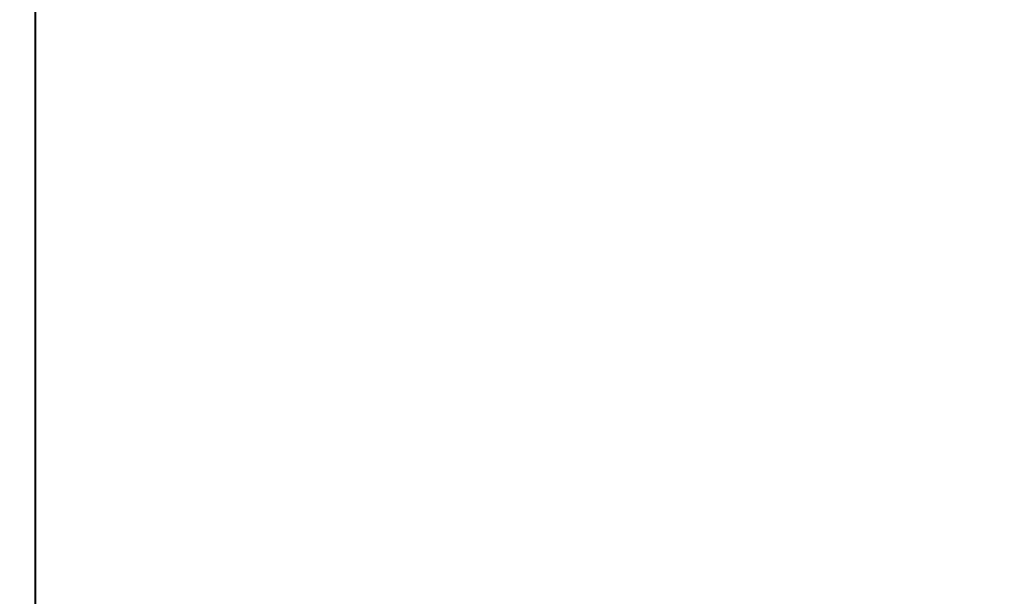
# Model space of a CAD drawing. Units: inches. Extents: x 459864 to 460310, y 324185 to 324787.
# Tile 83 of 112: x 460247.114882 to 460247.117712, y 324283.483832 to 324283.485489. Entities that reach past the tile are written whole.
import ezdxf

# ---------------------------------------------------------------- set-up
doc = ezdxf.new("R2010")
doc.units = ezdxf.units.IN
doc.layers.add('A-ANNO-DIMS', color=2, linetype='Continuous', lineweight=18)
doc.layers.add('A-WALL', color=7, linetype='Continuous', lineweight=40)
doc.styles.get("Standard").update_dxf_attribs({"font": 'arial.ttf'})
doc.dimstyles.new('ISO-25', dxfattribs={"dimtxt": 6, "dimasz": 2.5, "dimexe": 1.25, "dimexo": 0.625, "dimtad": 1, "dimdec": 1, "dimlunit": 3, "dimtxsty": 'Standard', "dimcen": 2.5, "dimadec": 0, "dimazin": 0, "dimtfac": 1, "dimtdec": 1, "dimtmove": 0, "dimatfit": 3, "dimfxl": 1, "dimarcsym": 0})

# ---------------------------------------------------------------- blocks, each defined once
blk = doc.blocks.new('*D21')
at = {"layer": 'A-ANNO-DIMS', "color": 0, "lineweight": -2, "transparency": 16777216}
for p, q in [((460247.7399266, 324715.4832328), (460309.5803685, 324715.4832328)), ((460308.3303685, 324712.9832328), (460308.3303685, 324285.9832328)), ((460247.7399266, 324283.4832328), (460309.5803685, 324283.4832328))]:
    blk.add_line(p, q, dxfattribs=at)
at = {"layer": 'A-ANNO-DIMS', "color": 0, "transparency": 16777216}
for points in [[(460307.9137019, 324712.9832328), (460308.7470352, 324712.9832328), (460308.3303685, 324715.4832328)], [(460307.9137019, 324285.9832328), (460308.7470352, 324285.9832328), (460308.3303685, 324283.4832328)]]:
    blk.add_solid(points, dxfattribs=at)
at = {"layer": 'Defpoints', "color": 0, "transparency": 16777216}
for p in [(460247.1149266, 324715.4832328), (460247.1149266, 324283.4832328), (460308.3303685, 324283.4832328)]:
    blk.add_point(p, dxfattribs=at)
at = {"layer": 'A-ANNO-DIMS', "color": 0, "transparency": 16777216, "insert": (460304.6398842, 324499.4832328), "char_height": 6, "attachment_point": 5, "rotation": 90}
blk.add_mtext("36'", dxfattribs=at)
blk = doc.blocks.new('*D62')
at = {"layer": 'A-ANNO-DIMS', "color": 0, "lineweight": -2, "transparency": 16777216}
for p, q in [((460247.739927, 324332.73872), (460278.764927, 324332.73872)), ((460277.514927, 324330.23872), (460277.514927, 324285.983233)), ((460247.739927, 324283.483233), (460278.764927, 324283.483233))]:
    blk.add_line(p, q, dxfattribs=at)
at = {"layer": 'A-ANNO-DIMS', "color": 0, "transparency": 16777216}
for points in [[(460277.0982603, 324330.23872), (460277.9315937, 324330.23872), (460277.514927, 324332.73872)], [(460277.0982603, 324285.983233), (460277.9315937, 324285.983233), (460277.514927, 324283.483233)]]:
    blk.add_solid(points, dxfattribs=at)
at = {"layer": 'Defpoints', "color": 0, "transparency": 16777216}
for p in [(460247.114927, 324332.73872), (460247.114927, 324283.483233), (460277.514927, 324283.483233)]:
    blk.add_point(p, dxfattribs=at)
at = {"layer": 'A-ANNO-DIMS', "color": 0, "transparency": 16777216, "insert": (460273.7876078, 324308.1109765), "char_height": 6, "attachment_point": 5, "rotation": 90}
blk.add_mtext('4\'-1 1/2"', dxfattribs=at)
blk = doc.blocks.new('*D67')
at = {"layer": 'A-ANNO-DIMS', "color": 0, "lineweight": -2, "transparency": 16777216}
for p, q in [((460208.114927, 324284.108233), (460208.114927, 324315.133233)), ((460247.114927, 324284.108233), (460247.114927, 324315.133233)), ((460210.614927, 324313.883233), (460244.614927, 324313.883233))]:
    blk.add_line(p, q, dxfattribs=at)
at = {"layer": 'A-ANNO-DIMS', "color": 0, "transparency": 16777216}
for points in [[(460210.614927, 324314.2998997), (460210.614927, 324313.4665663), (460208.114927, 324313.883233)], [(460244.614927, 324314.2998997), (460244.614927, 324313.4665663), (460247.114927, 324313.883233)]]:
    blk.add_solid(points, dxfattribs=at)
at = {"layer": 'Defpoints', "color": 0, "transparency": 16777216}
for p in [(460247.114927, 324313.883233), (460208.114927, 324283.483233), (460247.114927, 324283.483233)]:
    blk.add_point(p, dxfattribs=at)
at = {"layer": 'A-ANNO-DIMS', "color": 0, "transparency": 16777216, "insert": (460227.614927, 324317.5737173), "char_height": 6, "attachment_point": 5}
blk.add_mtext('3\'-3"', dxfattribs=at)

msp = doc.modelspace()

# ---------------------------------------------------------------- linework, layer by layer
at = {"layer": 'A-WALL'}
msp.add_line((460247.1149266, 324470.9832328), (460247.1149266, 324283.4832328), dxfattribs=at)

# ---------------------------------------------------------------- dimensions: what is measured, and where the dimension line sits
at = {"layer": 'A-ANNO-DIMS'}
for base, p1, p2, angle, override, picture, middle in [((460308.3303685, 324283.4832328), (460247.1149266, 324715.4832328), (460247.1149266, 324283.4832328), 90, {"dimclrd": 0, "dimclre": 0, "dimclrt": 0}, '*D21', (460304.6398842, 324499.4832328)), ((460277.514927, 324283.483233), (460247.114927, 324332.73872), (460247.114927, 324283.483233), 270, {"dimdec": 1, "dimlfac": 1, "dimrnd": 0, "dimzin": 1, "dimdsep": 46, "dimlunit": 4, "dimfrac": 2}, '*D62', (460273.7876078, 324308.1109765))]:
    dim = msp.add_linear_dim(base=base, p1=p1, p2=p2, angle=angle, dimstyle='ISO-25', override=override, dxfattribs=at)
    dim.commit()
    dim.dimension.update_dxf_attribs({"geometry": picture, "text_midpoint": middle})
dim = msp.add_linear_dim(base=(460247.114927, 324313.883233), p1=(460208.114927, 324283.483233), p2=(460247.114927, 324283.483233), dimstyle='ISO-25', override={"dimdec": 1, "dimlfac": 1, "dimrnd": 0, "dimzin": 1, "dimdsep": 46, "dimlunit": 4, "dimfrac": 2}, dxfattribs=at)
dim.commit()
dim.dimension.update_dxf_attribs({"geometry": '*D67', "text_midpoint": (460227.614927, 324317.5737173)})

doc.saveas('drawing.dxf')
